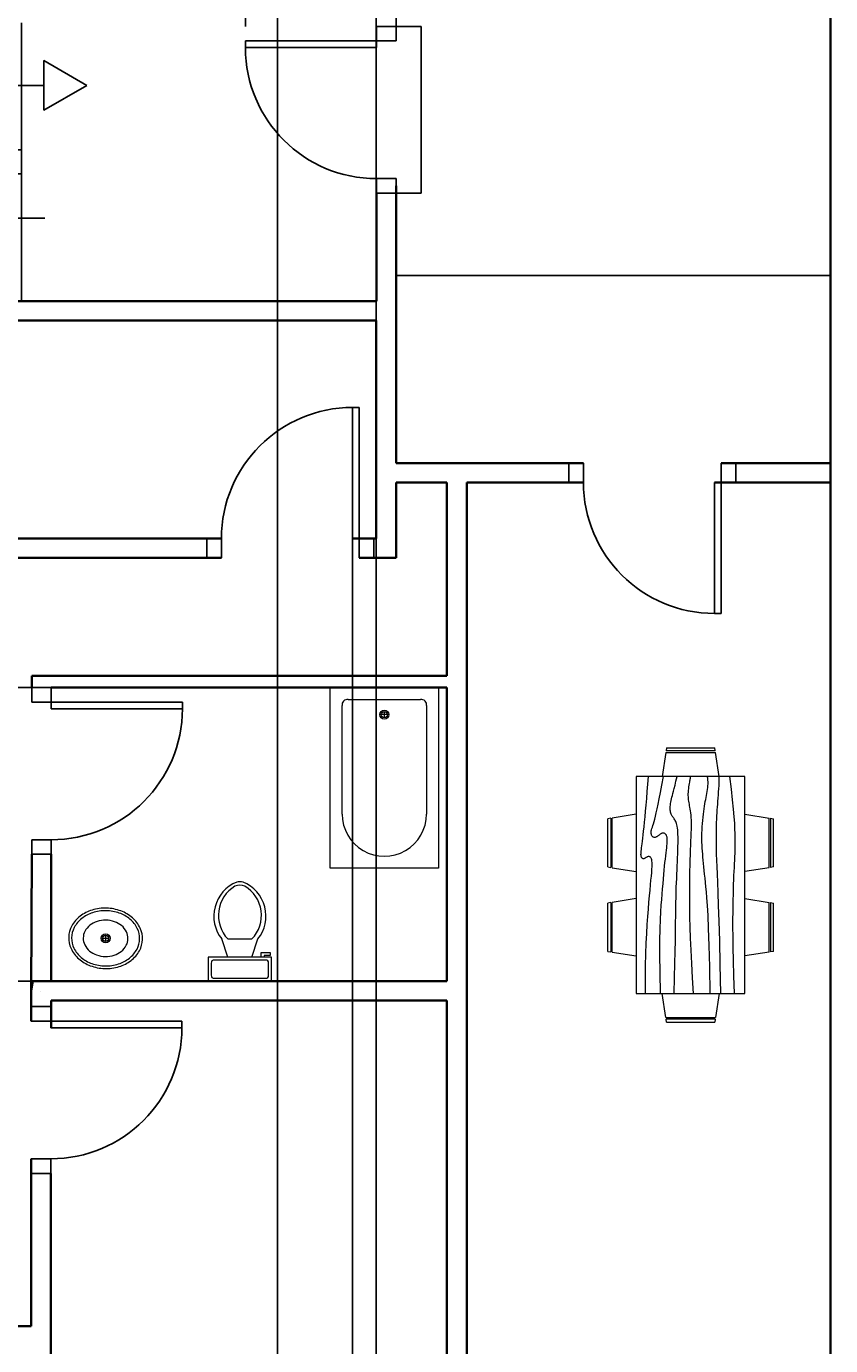
# Model space of a CAD drawing. Units: millimetres. Extents: x 31 to 27050, y -916 to 32407.
# Tile 3 of 7: x 6569 to 13341, y 5664 to 16782. Entities that reach past the tile are written whole.
import ezdxf

# ---------------------------------------------------------------- set-up
doc = ezdxf.new("R2010")
doc.units = ezdxf.units.MM
for name, color, linetype, lineweight in [('A-ANNO-DIMS', 2, 'Continuous', 18), ('A-DOOR', 3, 'Continuous', 25), ('A-FLOR-FIXT', 9, 'Continuous', 18), ('A-FLOR-STRS', 7, 'Continuous', 25), ('A-FURN', 8, 'Continuous', 13), ('A-WALL', 7, 'Continuous', 35)]:
    doc.layers.add(name, color=color, linetype=linetype, lineweight=lineweight)
doc.styles.get("Standard").update_dxf_attribs({"font": 'arial.ttf'})
doc.dimstyles.get("Standard").update_dxf_attribs({"dimtxt": 0.18, "dimasz": 0.18, "dimexe": 0.18, "dimexo": 0.0625, "dimgap": 0.09, "dimtad": 0, "dimtih": 1, "dimtoh": 1, "dimdec": 4, "dimzin": 0, "dimdsep": 46, "dimtxsty": 'Standard', "dimcen": 0.09, "dimadec": 0, "dimazin": 0, "dimtfac": 1, "dimtdec": 4, "dimtofl": 0, "dimtmove": 0, "dimatfit": 3, "dimfxl": 1, "dimtolj": 1, "dimtzin": 0, "dimarcsym": 0})

# ---------------------------------------------------------------- blocks, each defined once
blk = doc.blocks.new('Bath Tub - 26 x 60 in.')
for p, q in [((9, -17), (9, -19)), ((8, -18), (10, -18))]:
    blk.add_line(p, q)
blk.add_lwpolyline([(0, -36), (0, 0), (60, 0), (60, -36)], close=True)
for points in [[(6, -4), (42, -4)], [(4, -30), (4, -6)], [(42, -32), (6, -32)]]:
    blk.add_lwpolyline(points)
for radius in [1.5, 1]:
    blk.add_circle((9, -18), radius)
for centre, radius, start, end in [((5.75, -5.75), 1.767766999999999, 81.86989999999999, 188.1301), ((42, -18), 14, 270, 90), ((5.75, -30.25), 1.767766999999999, 171.8699, 278.1301)]:
    blk.add_arc(centre, radius, start, end)
blk = doc.blocks.new('Sink - Oval top')
for p, q in [((-1, 0), (1, 0)), ((0, 1), (0, -1))]:
    blk.add_line(p, q)
for points in [[(-12.23371880354079, 0.3941914712607968, 0.1176342565883263), (-11.46456229543957, -3.361933235489118, 0.104469279667093), (-8.878748691070427, -6.803541973650567, 0.0900157896014849), (-5.082757700676665, -9.072309807490512, 0.0819199491592185), (-0.3227280122732736, -10.01585280257211, 0.0819199491592091), (4.488169920880977, -9.380701564817912, 0.0900157896014801), (8.422342359155778, -7.36101289847943, 0.1044692796670922), (11.22435122606941, -4.093009071543406, 0.1176342565883338), (12.23371880354091, -0.3941914712607968, 0.1176342565883057), (11.46456229543992, 3.361933235488777, 0.1044692796670849), (8.878748691070427, 6.803541973650567, 0.0900157896014884), (5.082757700676324, 9.072309807490681, 0.0819199491592058), (0.3227280122732736, 10.01585280257211, 0.081919949159207), (-4.488169920880864, 9.380701564817969, 0.0900157896014802), (-8.422342359155778, 7.36101289847943, 0.1044692796670951), (-11.22435122606919, 4.093009071543633, 0.1176342565883402)], [(-11.28627986850119, 0.1590597164737346, 0.1186217001864142), (-10.51590095791209, -3.253161772358112, 0.1046781721811095), (-8.071803350560115, -6.358618019863342, 0.0895620664691738), (-4.537699193222351, -8.366971929609804, 0.0811846988912177), (-0.1289739026695997, -9.15150355811437, 0.0811846988912276), (4.300109150126218, -8.491524865184601, 0.0895620664691798), (7.889406708212618, -6.583562428127606, 0.1046781721811044), (10.42004782883111, -3.548216131892445, 0.1186217001864013), (11.28627986850119, -0.1590597164736209, 0.1186217001863945), (10.51590095791221, 3.253161772357998, 0.1046781721811069), (8.071803350560115, 6.358618019863342, 0.0895620664691756), (4.537699193222124, 8.366971929609917, 0.081184698891216), (0.1289739026695997, 9.151503558114428, 0.0811846988912142), (-4.300109150125877, 8.491524865184829, 0.0895620664691747), (-7.889406708212618, 6.583562428127606, 0.1046781721811045), (-10.42004782883111, 3.548216131892445, 0.1186217001863946)], [(-7.420452389032902, 0.0829876781601797, 0.1182825673856775), (-6.907065465214486, -2.1674649380775, 0.1046074595377274), (-5.294791470712084, -4.209988192029413, 0.0897179636260996), (-2.966599981142508, -5.528122152688069, 0.0814360825277113), (-0.0675135187855176, -6.036810076758797, 0.0814360825277218), (2.84222437824053, -5.593085960977873, 0.0897179636261315), (5.199312936802016, -4.327350491993342, 0.1046074595376878), (6.85686365682659, -2.321395784920355, 0.1182825673856714), (7.420452389033016, -0.0829876781601797, 0.1182825673856961), (6.907065465214486, 2.167464938077614, 0.1046074595377135), (5.294791470712084, 4.209988192029413, 0.0897179636261265), (2.966599981142621, 5.528122152687842, 0.0814360825277426), (0.0675135187855176, 6.036810076758797, 0.0814360825277225), (-2.842224378240644, 5.593085960977873, 0.0897179636261212), (-5.199312936802016, 4.327350491993342, 0.1046074595377049), (-6.856863656826476, 2.321395784920355, 0.1182825673856712)]]:
    blk.add_lwpolyline(points, format="xyb", close=True)
for radius in [1.5, 1]:
    blk.add_circle((0, 0), radius)
blk = doc.blocks.new('Toilet - top')
for p, q in [((9.5, -6), (9.5, -2)), ((-10, -8.5), (-8, -8.5)), ((-10, -9.5), (-10, -8.5)), ((-8, -8.5), (-8, -8)), ((-7, -8), (-7, -9.5)), ((-4, -8), (-6, -14)), ((4, -8), (6, -14)), ((-7, -9.5), (-10, -9.5)), ((4, -14), (-4, -14))]:
    blk.add_line(p, q)
blk.add_lwpolyline([(10.5, -8), (10.5, 0), (-10.5, 0), (-10.5, -8)], close=True)
for points in [[(-9.5, -2), (-9.5, -6)], [(8.5, -1), (-8.5, -1)], [(-8.5, -7), (8.5, -7)]]:
    blk.add_lwpolyline(points)
for centre, radius, start, end in [((-8.625, -1.875), 0.8838834999999999, 81.86989999999999, 188.1301), ((8.625, -1.875), 0.8838834999999999, 351.8699, 98.13009999999998), ((-8.625, -6.125), 0.8838834999999999, 171.869898, 278.1301), ((8.625, -6.125), 0.8838834999999999, 261.8699, 8.130099999999993), ((3.519562435188956, -21.58049502388982), 12.16902005083646, 141.4691096810948, 247.9714346835576), ((4.199957580658807, -21.81740929088453), 11.3291791325804, 136.3677254423718, 238.946823937405), ((-3.519499936778316, -21.58047137067522), 12.16903423757823, 292.0284332733152, 38.53070636800453), ((-4.199890672038477, -21.81738596564128), 11.32918622148567, 301.0530065773863, 43.63209216694732), ((2.09660981727e-05, -27.87646475467881), 4, 245.7318247449371, 294.2681740488959), ((2.09415214183e-05, -28.99996806116075), 4, 254.8605283244437, 285.1394707718433)]:
    blk.add_arc(centre, radius, start, end)
blk = doc.blocks.new('Dining Set - 36 x 72 in.')
for p, q in [((-22, 27.5), (-22.15620000000001, 26.50042)), ((-5.841600000000028, 26.5), (-22.15340000000003, 26.5)), ((-22, 27.5), (-6, 27.5)), ((-5.843700000000012, 26.49966), (-6, 27.5)), ((6, 27.5), (5.843799999999987, 26.50042)), ((22.15839999999997, 26.5), (5.846599999999966, 26.5)), ((6, 27.5), (22, 27.5)), ((22.15629999999999, 26.49966), (22, 27.5)), ((-22.23430000000002, 26.00059), (-23.48470000000003, 17.99762)), ((-22.23040000000003, 26), (-5.760800000000017, 26)), ((-4.515199999999992, 17.99762), (-5.765500000000031, 25.99926)), ((5.765699999999981, 26.00059), (4.515299999999967, 17.99762)), ((5.769599999999968, 26), (22.23919999999998, 26)), ((23.48480000000001, 17.99762), (22.23449999999997, 25.99926)), ((36, 18), (-36, 18)), ((-36, 18), (-36, -18)), ((36, -18), (36, 18)), ((-44.00060000000002, 8.234280000000002), (-35.99760000000003, 9.484740000000006)), ((44.00059999999996, 8.234280000000002), (35.99759999999998, 9.484740000000006)), ((-45.49999999999999, 8.000000000000004), (-44.50040000000001, 8.156170000000007)), ((-45.49999999999999, 8.000000000000004), (-45.49999999999999, -7.999999999999996)), ((-44.5, -8.15843), (-44.5, 8.153380000000002)), ((-44, 8.230410000000003), (-44, -8.239149999999999)), ((44, 8.230410000000003), (44, -8.239149999999999)), ((44.5, -8.15843), (44.5, 8.153380000000002)), ((45.49999999999999, 8.000000000000004), (44.50049999999999, 8.156170000000007)), ((45.49999999999999, 8.000000000000004), (45.49999999999999, -7.999999999999996)), ((-44.49970000000002, -8.156309999999994), (-45.49999999999999, -7.999999999999996)), ((-35.99760000000003, -9.484759999999998), (-43.9993, -8.234499999999993)), ((35.99759999999998, -9.484759999999998), (43.9993, -8.234499999999993)), ((44.49969999999995, -8.156309999999994), (45.49999999999999, -7.999999999999996)), ((-36, -18), (36, -18)), ((-22.23430000000002, -26.0006), (-23.48470000000003, -17.99762)), ((-4.515199999999992, -17.99762), (-5.765500000000031, -25.99928)), ((5.765699999999981, -26.0006), (4.515299999999967, -17.99762)), ((23.48480000000001, -17.99762), (22.23449999999997, -25.99928)), ((-22.23040000000003, -26), (-5.760800000000017, -26)), ((5.769599999999968, -26), (22.23919999999998, -26)), ((-22, -27.5), (-22.15620000000001, -26.50044)), ((-5.841600000000028, -26.5), (-22.15340000000003, -26.5)), ((-22, -27.5), (-6, -27.5)), ((-5.843700000000012, -26.49967), (-6, -27.5)), ((6, -27.5), (5.843799999999987, -26.50044)), ((22.15839999999997, -26.5), (5.846599999999966, -26.5)), ((6, -27.5), (22, -27.5)), ((22.15629999999999, -26.49967), (22, -27.5))]:
    blk.add_line(p, q)
for points in [[(-36, 15), (-31.17720000000003, 14.97754), (-26.80790000000002, 14.91406), (-22.85380000000003, 14.81543), (-19.27600000000001, 14.6875), (-16.03620000000001, 14.53613), (-13.09570000000002, 14.36718), (-10.41590000000002, 14.18652), (-7.958300000000008, 14), (-5.690400000000011, 13.81315), (-3.603499999999996, 13.63021), (-1.695400000000006, 13.45508), (0.0364999999999896, 13.29166), (1.594499999999982, 13.14388), (2.981099999999969, 13.01562), (4.198800000000005, 12.9108), (5.25, 12.83333), (6.139299999999991, 12.78613), (6.880200000000002, 12.76823), (7.488299999999981, 12.77767), (7.979199999999991, 12.8125), (8.368499999999983, 12.87077), (8.671899999999994, 12.95052), (8.904899999999998, 13.0498), (9.083300000000008, 13.16666), (9.220499999999959, 13.29899000000001), (9.32159999999999, 13.44401), (9.389499999999998, 13.59879), (9.427099999999996, 13.76041), (9.437299999999993, 13.92594), (9.423200000000008, 14.09245), (9.387499999999989, 14.257), (9.333300000000008, 14.41666), (9.263800000000003, 14.56917), (9.183600000000013, 14.71484), (9.097499999999968, 14.85465), (9.010400000000004, 14.98958), (8.92719999999997, 15.12060000000001), (8.852899999999975, 15.2487), (8.79219999999998, 15.37483), (8.75, 15.5), (8.730500000000006, 15.62467), (8.734399999999994, 15.74739), (8.761699999999962, 15.86621), (8.8125, 15.97916), (8.886699999999962, 16.08431), (8.984399999999994, 16.17968), (9.105500000000006, 16.26334), (9.25, 16.33333), (9.418900000000008, 16.38802), (9.617199999999968, 16.42708), (9.850599999999986, 16.45052), (10.125, 16.45833), (10.44630000000001, 16.45052), (10.82029999999997, 16.42708), (11.25290000000001, 16.38802), (11.75, 16.33333), (12.3184, 16.26318), (12.96940000000001, 16.17838), (13.7151, 16.07991), (14.5677, 15.96875), (15.53949999999997, 15.84586), (16.64259999999996, 15.71224), (17.88929999999999, 15.56884), (19.29169999999999, 15.41666), (20.85899999999998, 15.25667), (22.58789999999999, 15.08984), (24.47210000000001, 14.91715), (26.5052, 14.73958), (28.68090000000001, 14.5581), (30.99289999999996, 14.3737), (33.43469999999996, 14.18733), (36, 14)], [(-36, 10), (-28.97660000000002, 10.14274000000001), (-23.17250000000001, 10.20442), (-18.42410000000001, 10.19775), (-14.5677, 10.13541), (-11.43990000000002, 10.03011), (-8.87700000000001, 9.894530000000007), (-6.715399999999988, 9.741370000000005), (-4.791699999999991, 9.58333), (-2.96980000000002, 9.43082), (-1.224600000000009, 9.285150000000005), (0.4414999999999623, 9.14534), (2.02600000000001, 9.010410000000004), (3.526599999999973, 8.879390000000004), (4.940799999999967, 8.751300000000004), (6.265999999999962, 8.625160000000005), (7.5, 8.500000000000004), (8.641099999999994, 8.375490000000003), (9.691399999999987, 8.253900000000005), (10.65379999999999, 8.13818), (11.53120000000001, 8.031250000000004), (12.32669999999996, 7.936030000000005), (13.043, 7.85547), (13.68309999999997, 7.792480000000001), (14.25, 7.750000000000003), (14.74709999999999, 7.730300000000003), (15.17969999999997, 7.733070000000001), (15.55369999999999, 7.757320000000003), (15.875, 7.80208), (16.14940000000001, 7.866370000000006), (16.38279999999997, 7.94922), (16.58109999999999, 8.04964), (16.75, 8.166660000000004), (16.89439999999996, 8.29915), (17.01429999999999, 8.445310000000003), (17.1089, 8.603190000000001), (17.17709999999999, 8.77083), (17.21799999999996, 8.946290000000001), (17.2305, 9.127600000000005), (17.21369999999996, 9.312820000000006), (17.16669999999999, 9.500000000000004), (17.08949999999999, 9.687500000000004), (16.98699999999996, 9.875000000000004), (16.86489999999998, 10.0625), (16.72919999999999, 10.25), (16.5856, 10.4375), (16.44009999999997, 10.625), (16.29849999999999, 10.8125), (16.16669999999999, 11), (16.05000000000001, 11.18733), (15.95179999999999, 11.3737), (15.8752, 11.5581), (15.8229, 11.73958), (15.798, 11.91715), (15.80340000000001, 12.08984), (15.84199999999998, 12.25667), (15.91669999999999, 12.41666), (16.02949999999998, 12.56836), (16.17840000000001, 12.70833), (16.3605, 12.83268), (16.5729, 12.9375), (16.8127, 13.01888000000001), (17.07679999999999, 13.07291), (17.36250000000001, 13.0957), (17.66669999999999, 13.08333), (17.98939999999999, 13.03312), (18.34179999999998, 12.94726), (18.7382, 12.82918), (19.1927, 12.68229), (19.71949999999998, 12.51001), (20.33269999999999, 12.31575), (21.04649999999998, 12.10294), (21.875, 11.875), (22.83569999999997, 11.63354), (23.95900000000001, 11.37304), (25.27859999999999, 11.08618), (26.82819999999998, 10.76562), (28.64139999999998, 10.40405), (30.75200000000001, 9.994140000000005), (33.1936, 9.528560000000002), (36, 9.000000000000004)], [(-36, 5.500000000000003), (-30.71570000000003, 5.334800000000004), (-26.06900000000002, 5.20963), (-21.99459999999999, 5.11767), (-18.42709999999999, 5.05208), (-15.30090000000001, 5.006020000000003), (-12.55080000000004, 4.972650000000005), (-10.1112, 4.945150000000001), (-7.916699999999991, 4.916660000000003), (-5.908999999999991, 4.881670000000003), (-4.058600000000012, 4.839840000000005), (-2.342899999999985, 4.792150000000003), (-0.7395999999999959, 4.73958), (0.7738999999999692, 4.683100000000006), (2.21999999999997, 4.623700000000003), (3.621299999999962, 4.562330000000006), (5, 4.500000000000003), (6.37299999999999, 4.437820000000005), (7.734399999999993, 4.377600000000004), (9.072299999999984, 4.321290000000001), (10.375, 4.27083), (11.63089999999999, 4.228190000000001), (12.8281, 4.195310000000002), (13.95509999999996, 4.17415), (15, 4.166660000000003), (15.95400000000001, 4.174480000000006), (16.81899999999996, 4.197910000000003), (17.6001, 4.236980000000006), (18.30209999999999, 4.291660000000003), (18.92989999999997, 4.361980000000006), (19.48829999999998, 4.447910000000003), (19.98230000000001, 4.549480000000006), (20.41669999999999, 4.666660000000003), (20.79689999999999, 4.798990000000006), (21.1302, 4.944010000000002), (21.42449999999997, 5.098790000000004), (21.6875, 5.260410000000003), (21.92709999999999, 5.42594), (22.15109999999999, 5.592450000000003), (22.36719999999997, 5.757000000000001), (22.58339999999998, 5.916660000000003), (22.80649999999997, 6.068680000000004), (23.04039999999998, 6.210930000000001), (23.28789999999998, 6.341470000000004), (23.5521, 6.45833), (23.83580000000001, 6.559570000000004), (24.142, 6.643230000000006), (24.4735, 6.707350000000001), (24.83339999999998, 6.750000000000003), (25.2235, 6.76969), (25.642, 6.766920000000002), (26.08580000000001, 6.74267), (26.5521, 6.697910000000003), (27.03789999999998, 6.633620000000004), (27.54039999999998, 6.550780000000006), (28.05649999999997, 6.450360000000006), (28.58339999999998, 6.33333), (29.12419999999997, 6.19987), (29.70709999999997, 6.046870000000001), (30.36609999999996, 5.870440000000005), (31.1354, 5.666660000000003), (32.04929999999996, 5.431640000000005), (33.142, 5.161460000000001), (34.44749999999999, 4.852210000000003), (36, 4.500000000000003)], [(-36, -0.9999999999999964), (-30.79150000000004, -0.6590999999999987), (-26.01949999999999, -0.3821599999999954), (-21.65190000000001, -0.1628399999999992), (-17.65629999999999, 0.0052100000000017), (-14.00049999999999, 0.1283300000000018), (-10.65230000000002, 0.2128900000000051), (-7.579600000000027, 0.2652200000000029), (-4.75, 0.2916600000000038), (-2.134000000000014, 0.2979300000000045), (0.2878000000000043, 0.287110000000002), (2.5317, 0.2616300000000002), (4.614599999999995, 0.2239600000000017), (6.552899999999965, 0.1765100000000039), (8.363299999999981, 0.1217400000000062), (10.06229999999999, 0.0620900000000013), (11.66669999999999, 3.6e-15), (13.18989999999996, -0.0620099999999972), (14.63409999999999, -0.1210999999999949), (15.9982, -0.174319999999998), (17.28129999999999, -0.2187499999999964), (18.48230000000001, -0.2514699999999941), (19.6003, -0.2695299999999996), (20.6343, -0.2700199999999988), (21.58339999999999, -0.2499999999999964), (22.44810000000001, -0.2076799999999999), (23.23570000000001, -0.1458399999999962), (23.95490000000001, -0.0683599999999949), (24.6146, 0.0208300000000001), (25.2235, 0.1178400000000046), (25.79039999999998, 0.2187500000000035), (26.32409999999999, 0.3196600000000025), (26.83339999999998, 0.4166600000000038), (27.32650000000001, 0.5061800000000041), (27.80989999999997, 0.5859300000000012), (28.2894, 0.6539700000000046), (28.77089999999999, 0.7083300000000002), (29.26009999999997, 0.7470700000000045), (29.76299999999998, 0.7682300000000062), (30.28550000000001, 0.7698500000000017), (30.83339999999998, 0.7500000000000036), (31.40879999999999, 0.707840000000001), (31.99939999999998, 0.6471300000000006), (32.589, 0.5727500000000028), (33.16149999999999, 0.4895800000000002), (33.70079999999996, 0.402500000000007), (34.19079999999997, 0.3164000000000051), (34.61529999999999, 0.2361600000000017), (34.95839999999998, 0.1666600000000038), (35.20990000000001, 0.1116500000000009), (35.38479999999998, 0.0703100000000028), (35.50399999999996, 0.0406900000000015), (35.58859999999999, 0.0208300000000001), (35.65940000000001, 0.0087900000000012), (35.73769999999996, 0.0026000000000046), (35.8442, 0.0003200000000056), (36, 3.6e-15)], [(-36, -6.499999999999996), (-27.18430000000001, -6.312669999999993), (-20.084, -6.126299999999996), (-14.46899999999999, -5.941899999999993), (-10.10939999999999, -5.760419999999999), (-6.77520000000004, -5.582849999999996), (-4.236300000000028, -5.410159999999994), (-2.262900000000001, -5.243329999999996), (-0.625, -5.083339999999996), (0.8707999999999742, -4.930989999999997), (2.271500000000003, -4.786459999999994), (3.587199999999995, -4.649739999999997), (4.828100000000006, -4.520839999999996), (6.004599999999982, -4.399739999999997), (7.127000000000009, -4.286459999999994), (8.205299999999966, -4.180989999999997), (9.25, -4.083339999999996), (10.27049999999997, -3.993819999999995), (11.27339999999998, -3.914069999999998), (12.2647, -3.846029999999995), (13.25, -3.791669999999999), (14.23539999999997, -3.752929999999995), (15.22659999999996, -3.731769999999993), (16.22949999999997, -3.730149999999998), (17.25, -3.749999999999996), (18.2912, -3.792479999999994), (19.3451, -3.855469999999993), (20.40089999999998, -3.936039999999994), (21.4479, -4.031249999999996), (22.47539999999998, -4.138189999999998), (23.47269999999998, -4.253909999999994), (24.4289, -4.375489999999995), (25.33339999999999, -4.499999999999996), (26.17849999999999, -4.624919999999999), (26.96940000000001, -4.749349999999996), (27.71449999999999, -4.872809999999997), (28.4219, -4.994789999999998), (29.09999999999996, -5.114829999999994), (29.75720000000001, -5.232419999999994), (30.40159999999997, -5.347089999999997), (31.04169999999999, -5.458339999999996), (31.68369999999999, -5.564369999999993), (32.32619999999997, -5.658209999999993), (32.9658, -5.731529999999995), (33.59899999999999, -5.776039999999998), (34.22239999999999, -5.783449999999998), (34.83269999999999, -5.745449999999994), (35.4264, -5.653729999999999), (36, -5.499999999999996)], [(-36, -9.999999999999996), (-26.40219999999999, -9.812989999999996), (-18.46750000000003, -9.628909999999994), (-11.9839, -9.450689999999998), (-6.739599999999995, -9.281249999999996), (-2.522600000000011, -9.123539999999995), (0.8788999999999872, -8.980469999999993), (3.676899999999989, -8.854979999999994), (6.083300000000008, -8.749999999999996), (8.276700000000005, -8.667649999999998), (10.30209999999999, -8.606769999999994), (12.1712, -8.565429999999996), (13.89580000000001, -8.54167), (15.48759999999998, -8.533529999999995), (16.95830000000001, -8.539069999999999), (18.31970000000001, -8.556319999999994), (19.58339999999998, -8.583339999999996), (20.76159999999999, -8.618409999999994), (21.86849999999998, -8.660809999999994), (22.91879999999998, -8.710039999999996), (23.9271, -8.765629999999998), (24.90809999999999, -8.827069999999996), (25.87629999999996, -8.89388), (26.84649999999999, -8.96558), (27.83339999999999, -9.04167), (28.84739999999999, -9.121179999999997), (29.88279999999998, -9.201169999999994), (30.93000000000001, -9.278239999999993), (31.97919999999999, -9.348959999999995), (33.02049999999997, -9.409909999999998), (34.04429999999996, -9.45768), (35.04069999999996, -9.488849999999996), (36, -9.499999999999996)], [(-36, -14.5), (-30.0881, -14.33512999999999), (-25.03320000000002, -14.21224), (-20.7312, -14.12646999999999), (-17.0781, -14.07292), (-13.97000000000003, -14.04670999999999), (-11.30270000000001, -14.04296999999999), (-8.972399999999993, -14.05680999999999), (-6.875, -14.08333999999999), (-4.922400000000038, -14.11832999999999), (-3.09050000000002, -14.16015999999999), (-1.370900000000006, -14.20784999999999), (0.2447999999999979, -14.26042), (1.764700000000004, -14.31689999999999), (3.197299999999984, -14.37629999999999), (4.550700000000006, -14.43766999999999), (5.833300000000008, -14.5), (7.055399999999963, -14.5621), (8.235000000000014, -14.62174999999999), (9.392200000000003, -14.67652), (10.54689999999999, -14.72395999999999), (11.7192, -14.76164), (12.92899999999997, -14.78711), (14.19649999999996, -14.79794), (15.54169999999999, -14.79167), (16.99329999999998, -14.76423999999999), (18.61519999999996, -14.70508), (20.48039999999998, -14.60197), (22.66149999999999, -14.44270999999999), (25.2312, -14.21509), (28.26240000000002, -13.90689999999999), (31.8277, -13.50594), (36, -13)]]:
    blk.add_lwpolyline(points)
blk = doc.blocks.new('DOOR-SINGLE-1104')
for p, q in [((56.41678681898429, 1104.337341461596), (-7.18501e-11, 1104.337341461596)), ((-7.18501e-11, 1104.337341461596), (-7.18501e-11, 3.638e-12)), ((56.41678681898429, 7.276e-12), (56.41678681898429, 1104.337341461596)), ((-1226.913698425656, -163.8831223050438), (-1226.913698425656, 3.638e-12)), ((-1104.337341461589, 3.638e-12), (-1226.913698425656, 7.276e-12)), ((-1104.337341461589, 3.638e-12), (-1104.337341461589, -163.8831223050438)), ((-7.18501e-11, 3.638e-12), (56.41678681898429, 7.276e-12)), ((56.41678681898429, -163.8831223050438), (56.41678681898429, 3.638e-12)), ((56.41678681898429, 3.638e-12), (178.9931437830519, 3.638e-12)), ((178.9931437830519, 3.638e-12), (178.9931437830519, -163.8831223050438)), ((-1104.337341461589, -163.8831223050438), (-1226.913698425656, -163.8831223050438)), ((178.9931437830519, -163.8831223050438), (56.41678681898429, -163.8831223050438))]:
    blk.add_line(p, q)
blk.add_arc((0, 3.638e-12), 1104.337341461589, 90, 180)
blk = doc.blocks.new('STAIR-RETURN-2400')
for p, q in [((9.095e-13, 2345.636859649549), (9.095e-13, -1.819e-12)), ((200.0000000000009, 2345.636859649549), (200.0000000000009, -1.819e-12)), ((400.0000000000008, 2345.636859649549), (400.0000000000008, -1.819e-12)), ((600.0000000000008, 2345.636859649549), (600.0000000000008, -1.819e-12)), ((800.0000000000008, 2345.636859649552), (800.0000000000008, 1.819e-12)), ((1000.000000000001, 2345.636859649556), (1000.000000000001, 5.457e-12)), ((1200.000000000001, 2345.636859649556), (1200.000000000001, 5.457e-12)), ((1400.000000000001, 2345.636859649556), (1400.000000000001, 5.457e-12)), ((1600.000000000001, 2345.636859649559), (1600.000000000001, 9.0949e-12)), ((1800.000000000001, 2345.636859649559), (1800.000000000001, 9.0949e-12)), ((2000.000000000001, 2345.636859649559), (2000.000000000001, 9.0949e-12)), ((2200.000000000001, 2345.636859649563), (2200.000000000001, 1.27329e-11)), ((2400.000000000001, 2345.636859649563), (2400.000000000001, 1.27329e-11)), ((-415.9249645337103, 697.4958917418807), (-415.9249645337103, 1817.654410237617)), ((-415.9249645337103, 1817.654410237617), (2588.331988211024, 1817.654410237617)), ((9.095e-13, 1172.818429824772), (9.095e-13, 1272.818429824772)), ((9.095e-13, 1272.818429824772), (2400.000000000001, 1272.818429824774)), ((2400.000000000001, 1272.818429824774), (2400.000000000001, 1072.818429824774)), ((2400.000000000001, 1072.818429824774), (9.095e-13, 1072.818429824774)), ((2597.09055342863, 697.4958917418807), (-415.9249645337103, 697.4958917418807))]:
    blk.add_line(p, q)
blk.add_lwpolyline([(2948.607295106225, 1817.654410237617), (2588.331988211024, 2025.65945565594), (2588.331988211024, 1609.649364819299)], close=True)
blk = doc.blocks.new('*D16')
at = {"layer": 'A-ANNO-DIMS', "color": 0, "lineweight": -2, "transparency": 16777216}
for p, q in [((9681.744557342236, 16781.90361905769), (9892.748083673547, 16781.90361905769)), ((9892.568083673546, 16781.72361905769), (9892.568083673546, 16079.13332892196)), ((9892.568083673546, 15376.17677684898), (9892.568083673546, 16078.76706698471)), ((9681.744557342237, 15375.99677684898), (9892.748083673547, 15375.99677684898))]:
    blk.add_line(p, q, dxfattribs=at)
at = {"layer": 'A-ANNO-DIMS', "color": 0, "transparency": 16777216}
for points in [[(9892.538083673546, 16781.72361905769), (9892.598083673547, 16781.72361905769), (9892.568083673546, 16781.90361905769)], [(9892.538083673546, 15376.17677684898), (9892.598083673547, 15376.17677684898), (9892.568083673546, 15375.99677684898)]]:
    blk.add_solid(points, dxfattribs=at)
at = {"layer": 'Defpoints', "color": 0, "transparency": 16777216}
for p in [(9681.682057342236, 16781.90361905769), (9892.568083673546, 16781.90361905769), (9681.682057342237, 15375.99677684898)]:
    blk.add_point(p, dxfattribs=at)
at = {"layer": 'A-ANNO-DIMS', "color": 0, "transparency": 16777216, "insert": (9892.568083673552, 16078.95019795333), "char_height": 0.18, "attachment_point": 5}
blk.add_mtext('\\A1;DOOR 1406 TYP.', dxfattribs=at)
blk = doc.blocks.new('*D17')
at = {"layer": 'A-ANNO-DIMS', "color": 0, "lineweight": -2, "transparency": 16777216}
for p, q in [((8413.461593575592, 16781.96611905768), (8413.461593575592, 16992.96964538898)), ((8413.641593575592, 16992.78964538898), (9046.912357518939, 16992.78964538899)), ((9681.502057342232, 16992.78964538899), (9048.231293398885, 16992.78964538899)), ((9681.682057342232, 16781.96611905768), (9681.682057342232, 16992.96964538899))]:
    blk.add_line(p, q, dxfattribs=at)
at = {"layer": 'A-ANNO-DIMS', "color": 0, "transparency": 16777216}
for points in [[(8413.641593575592, 16992.81964538898), (8413.641593575592, 16992.75964538898), (8413.461593575592, 16992.78964538898)], [(9681.502057342232, 16992.81964538899), (9681.502057342232, 16992.75964538899), (9681.682057342232, 16992.78964538899)]]:
    blk.add_solid(points, dxfattribs=at)
at = {"layer": 'Defpoints', "color": 0, "transparency": 16777216}
for p in [(8413.461593575592, 16992.78964538898), (8413.461593575592, 16781.90361905768), (9681.682057342232, 16781.90361905768)]:
    blk.add_point(p, dxfattribs=at)
at = {"layer": 'A-ANNO-DIMS', "color": 0, "transparency": 16777216, "insert": (9047.571825458914, 16992.78964538899), "char_height": 0.18, "attachment_point": 5}
blk.add_mtext('\\A1;1268 TYP.', dxfattribs=at)
blk = doc.blocks.new('*D64')
at = {"layer": 'A-ANNO-DIMS', "color": 0, "lineweight": -2, "transparency": 16777216}
for p, q in [((6778.040612000004, 11210.336516), (5198.923112000002, 11210.336516)), ((5199.103112000003, 11210.156516), (5199.103112000003, 9972.897271637792)), ((5199.103112000003, 8735.274221000001), (5199.103112000003, 9972.533465362214)), ((6778.040612000004, 8735.094221000001), (5198.923112000003, 8735.094221000001))]:
    blk.add_line(p, q, dxfattribs=at)
at = {"layer": 'A-ANNO-DIMS', "color": 0, "transparency": 16777216}
for points in [[(5199.073112000003, 11210.156516), (5199.133112000002, 11210.156516), (5199.103112000003, 11210.336516)], [(5199.073112000004, 8735.274221000001), (5199.133112000003, 8735.274221000001), (5199.103112000003, 8735.094221000001)]]:
    blk.add_solid(points, dxfattribs=at)
at = {"layer": 'Defpoints', "color": 0, "transparency": 16777216}
for p in [(5199.103112000003, 11210.336516), (6778.103112000003, 11210.336516), (6778.103112000003, 8735.094221000001)]:
    blk.add_point(p, dxfattribs=at)
at = {"layer": 'A-ANNO-DIMS', "color": 0, "transparency": 16777216, "insert": (5199.103112000005, 9972.7153685), "char_height": 0.18, "attachment_point": 5}
blk.add_mtext('\\A1;2475', dxfattribs=at)
blk = doc.blocks.new('*D68')
at = {"layer": 'A-ANNO-DIMS', "color": 0, "lineweight": -2, "transparency": 16777216}
for p, q in [((9681.682057000002, 13102.073129), (9681.682057000002, 14681.190629)), ((9681.862057, 14681.010629), (11510.77480004775, 14681.010629)), ((13340.405333, 14681.010629), (11511.49258995225, 14681.010629)), ((13340.585333, 13102.073129), (13340.585333, 14681.190629))]:
    blk.add_line(p, q, dxfattribs=at)
at = {"layer": 'A-ANNO-DIMS', "color": 0, "transparency": 16777216}
for points in [[(9681.862057, 14681.040629), (9681.862057, 14680.980629), (9681.682057000002, 14681.010629)], [(13340.405333, 14681.040629), (13340.405333, 14680.980629), (13340.585333, 14681.010629)]]:
    blk.add_solid(points, dxfattribs=at)
at = {"layer": 'Defpoints', "color": 0, "transparency": 16777216}
for p in [(13340.585333, 14681.010629), (9681.682057000002, 13102.010629), (13340.585333, 13102.010629)]:
    blk.add_point(p, dxfattribs=at)
at = {"layer": 'A-ANNO-DIMS', "color": 0, "transparency": 16777216, "insert": (11511.133695, 14681.010629), "char_height": 0.18, "attachment_point": 5}
blk.add_mtext('\\A1;3659', dxfattribs=at)
blk = doc.blocks.new('*D74')
at = {"layer": 'A-ANNO-DIMS', "color": 0, "lineweight": -2, "transparency": 16777216}
for p, q in [((8684.522829, 19025.373224), (8684.522828999998, -915.5318640000004)), ((9513.331407, 19025.373224), (9513.331407, -915.5318640000004)), ((8684.702829, -915.3518639999999), (9098.533107085947, -915.3518639999999)), ((9513.151406999998, -915.3518639999999), (9099.321128914047, -915.3518639999999))]:
    blk.add_line(p, q, dxfattribs=at)
at = {"layer": 'A-ANNO-DIMS', "color": 0, "transparency": 16777216}
for points in [[(8684.702829, -915.321864), (8684.702829, -915.381864), (8684.522828999998, -915.3518639999999)], [(9513.151406999998, -915.321864), (9513.151406999998, -915.381864), (9513.331407, -915.3518639999999)]]:
    blk.add_solid(points, dxfattribs=at)
at = {"layer": 'Defpoints', "color": 0, "transparency": 16777216}
for p in [(8684.522829, 19025.435724), (9513.331407, 19025.435724), (8684.522828999998, -915.3518639999999)]:
    blk.add_point(p, dxfattribs=at)
at = {"layer": 'A-ANNO-DIMS', "color": 0, "transparency": 16777216, "insert": (9098.927117999998, -915.3518639999999), "char_height": 0.18, "attachment_point": 5}
blk.add_mtext('\\A1;828.8', dxfattribs=at)
blk = doc.blocks.new('*D75')
at = {"layer": 'A-ANNO-DIMS', "color": 0, "lineweight": -2, "transparency": 16777216}
for p, q in [((9315.42813, 12465.681171), (9315.42813, -915.5318640000004)), ((9513.331407, 12465.681171), (9513.331407, -915.5318640000004)), ((9315.60813, -915.3518639999999), (9413.994352401773, -915.3518639999999)), ((9513.151407, -915.3518639999999), (9414.765184598225, -915.3518639999999))]:
    blk.add_line(p, q, dxfattribs=at)
at = {"layer": 'A-ANNO-DIMS', "color": 0, "transparency": 16777216}
for points in [[(9315.60813, -915.321864), (9315.60813, -915.381864), (9315.42813, -915.3518639999999)], [(9513.151407, -915.321864), (9513.151407, -915.381864), (9513.331407, -915.3518639999999)]]:
    blk.add_solid(points, dxfattribs=at)
at = {"layer": 'Defpoints', "color": 0, "transparency": 16777216}
for p in [(9315.42813, 12465.743671), (9513.331407, 12465.743671), (9513.331407, -915.3518639999999)]:
    blk.add_point(p, dxfattribs=at)
at = {"layer": 'A-ANNO-DIMS', "color": 0, "transparency": 16777216, "insert": (9414.379768499999, -915.3518639999999), "char_height": 0.18, "attachment_point": 5}
blk.add_mtext('\\A1;197.9', dxfattribs=at)

msp = doc.modelspace()

# ---------------------------------------------------------------- linework, layer by layer
at = {"layer": 'A-DOOR'}
for p, q in [((6778.103112139866, 11210.33651640691), (6614.219989834819, 11210.33651640691)), ((6773.905119419517, 8521.175884980112), (6610.021997114469, 8521.175884980112))]:
    msp.add_line(p, q, dxfattribs=at)
at = {"layer": 'A-WALL'}
for p, q in [((13340.58533261045, 13102.01062910059), (13340.58533261045, 17938.12750679554)), ((9517.798935037174, 15375.99677684899), (9517.798935037174, 14467.4249367068)), ((9681.682057342221, 14467.4249367068), (9681.682057342221, 15437.28495533102)), ((2757.34083568836, 14467.4249367068), (9517.798935037174, 14467.4249367068)), ((9681.682057342221, 14384.27405581066), (9681.682057342221, 14467.4249367068)), ((9681.682057342221, 14384.27405581066), (9681.682057342221, 13102.01062910059)), ((2925.691486399059, 14303.54181440175), (9513.331406631527, 14303.54181440175)), ((9513.331406631527, 14303.54181440175), (9513.331406631527, 12465.74367114626)), ((11259.57994150526, 13102.01062910059), (9681.682057342221, 13102.01062910059)), ((13340.58533261045, 13102.01062910059), (12420.33406978584, 13102.01062910059)), ((13340.58533261045, 12938.12750679554), (13340.58533261045, 13102.01062910059)), ((9681.682057342221, 12938.12750679554), (9681.682057342221, 12382.59279025013)), ((10110.02199711447, 12938.12750679554), (9681.682057342221, 12938.12750679554)), ((10110.02199711447, 12938.12750679554), (10110.02199711446, 11309.00881926711)), ((10278.37264782516, 12938.12750679554), (10278.37264782516, 827.5312586717337)), ((11259.57994150526, 12938.12750679554), (10278.37264782516, 12938.12750679554)), ((13340.58533261045, 12938.12750679554), (12363.91728296678, 12938.12750679554)), ((13340.58533261045, 827.5312586717337), (13340.58533261045, 12938.12750679554)), ((8211.090788713413, 12465.74367114626), (2925.691486399059, 12465.74367114627)), ((9513.331406631527, 12465.74367114626), (9315.428130174929, 12465.74367114626)), ((9681.682057342221, 12301.86054884122), (9681.682057342221, 12382.59279025013)), ((8211.090788713413, 12301.86054884122), (5781.707676021313, 12301.86054884121)), ((9593.894742127508, 12301.86054884122), (9371.844916993983, 12301.86054884122)), ((9593.894742127508, 12301.86054884122), (9681.682057342221, 12301.86054884122)), ((6614.219989834819, 11210.33651640691), (6614.219989834819, 11309.00881926711)), ((6614.219989834819, 11309.00881926711), (10110.02199711447, 11309.00881926711)), ((6778.103112139866, 11210.33651640691), (10110.02199711447, 11210.33651640691)), ((10110.02199711447, 11210.33651640691), (10110.02199711447, 8735.094220936826)), ((6614.219989834822, 9804.429674198203), (6610.021997114469, 8651.943340040685)), ((6778.103112139874, 9804.429674198203), (6778.103112139874, 8735.094220936826)), ((6610.021997114469, 8651.943340040685), (6610.021997114469, 8735.094220936828)), ((6610.021997114469, 8735.094220936828), (6690.58533261045, 8735.094220936826)), ((6610.021997114469, 8651.943340040685), (6622.148902538111, 8735.094220936828)), ((6690.58533261045, 8735.094220936826), (10110.02199711447, 8735.094220936826)), ((6610.021997114469, 8398.599528016042), (6610.021997114469, 8651.943340040685)), ((6690.58533261045, 8651.943340040685), (6690.58533261045, 8651.943340040685)), ((6778.372647825162, 8571.211098631777), (10110.02199711446, 8571.211098631771)), ((6778.372647825162, 8342.182741196984), (6778.372647825162, 8571.211098631777)), ((10110.02199711447, 8571.211098631777), (10110.02199711447, 827.5312586717337)), ((6610.021997114469, 5827.531258671733), (6610.021997114471, 7237.845399735471)), ((6773.905119419524, 7115.269042771405), (6778.372647825162, 827.5312586717337)), ((6302.191350742941, 5827.531258671733), (6610.021997114469, 5827.531258671733))]:
    msp.add_line(p, q, dxfattribs=at)

# ---------------------------------------------------------------- block references
at = {"layer": 'A-DOOR', "rotation": 90.00000000000006}
msp.add_blockref('DOOR-SINGLE-1104', (9517.798935037188, 16602.91047527463), dxfattribs=at)
at = {"layer": 'A-DOOR'}
msp.add_blockref('DOOR-SINGLE-1104', (9315.428130175002, 12465.74367114624), dxfattribs=at)
at = {"layer": 'A-DOOR', "extrusion": (0, 0, -1), "zscale": -1}
for p, rotation in [((-12363.91728296685, 12938.12750679555), 180), ((-6778.103112139851, 11031.34337262386), 90.00000000000028), ((-6773.905119419501, 8342.182741197055), 89.99999999999996)]:
    msp.add_blockref('DOOR-SINGLE-1104', p, dxfattribs=dict(at, rotation=rotation))
at = {"layer": 'A-FLOR-FIXT', "xscale": 25.4, "yscale": 25.4, "zscale": 25.4}
for name, p, rotation in [('Bath Tub - 26 x 60 in.', (10040.2342069835, 11210.33651640691), 270), ('Toilet - top', (8366.84177489248, 8735.094220936826), 180)]:
    msp.add_blockref(name, p, dxfattribs=dict(at, rotation=rotation))
msp.add_blockref('Sink - Oval top', (7236.106883122694, 9096.171958548497), dxfattribs=at)
at = {"layer": 'A-FLOR-STRS'}
msp.add_blockref('STAIR-RETURN-2400', (4128.594056532892, 14467.4249367068), dxfattribs=at)
at = {"layer": 'A-FURN', "xscale": 25.4, "yscale": 25.4, "zscale": 25.4, "rotation": 90}
msp.add_blockref('Dining Set - 36 x 72 in.', (12162.05807908132, 9545.199603633526), dxfattribs=at)

# ---------------------------------------------------------------- dimensions: what is measured, and where the dimension line sits
at = {"layer": 'A-ANNO-DIMS'}
for base, p1, p2, override, picture, middle in [((8684.522828999998, -915.3518639999999), (9513.331407, 19025.435724), (8684.522829, 19025.435724), {"dimdec": 1, "dimlfac": 1, "dimrnd": 0, "dimzin": 0, "dimdsep": 46, "dimlunit": 2}, '*D74', (9098.927117999998, -915.3518639999999)), ((13340.585333, 14681.010629), (9681.682057000002, 13102.010629), (13340.585333, 13102.010629), {"dimdec": 0, "dimlfac": 1, "dimrnd": 0, "dimzin": 0, "dimdsep": 46, "dimlunit": 2}, '*D68', (11511.133695, 14681.010629)), ((9513.331407, -915.3518639999999), (9315.42813, 12465.743671), (9513.331407, 12465.743671), {"dimdec": 1, "dimlfac": 1, "dimrnd": 0, "dimzin": 0, "dimdsep": 46, "dimlunit": 2}, '*D75', (9414.379768499999, -915.3518639999999))]:
    dim = msp.add_linear_dim(base=base, p1=p1, p2=p2, dimstyle='Standard', override=override, dxfattribs=at)
    dim.commit()
    dim.dimension.update_dxf_attribs({"geometry": picture, "text_midpoint": middle})
for base, p1, p2, angle, text, picture, middle in [((8413.461593575592, 16992.78964538898), (9681.682057342232, 16781.90361905768), (8413.461593575592, 16781.90361905768), 180.0000000000001, '<> TYP.', '*D17', (9047.571825458914, 16992.78964538899)), ((9892.568083673546, 16781.90361905769), (9681.682057342234, 15375.99677684897), (9681.682057342232, 16781.90361905768), 90.00000000000007, 'DOOR <> TYP.', '*D16', (9892.568083673552, 16078.95019795333))]:
    dim = msp.add_linear_dim(base=base, p1=p1, p2=p2, angle=angle, text=text, dimstyle='Standard', override={"dimdec": 0, "dimlfac": 1, "dimrnd": 0, "dimzin": 0, "dimdsep": 46, "dimlunit": 2}, dxfattribs=at)
    dim.commit()
    dim.dimension.update_dxf_attribs({"geometry": picture, "text_midpoint": middle})
dim = msp.add_linear_dim(base=(5199.103112000003, 11210.336516), p1=(6778.103112, 8735.094221), p2=(6778.103112, 11210.336516), angle=90.00000000000018, dimstyle='Standard', override={"dimdec": 0, "dimlfac": 1, "dimrnd": 0, "dimzin": 0, "dimdsep": 46, "dimlunit": 2}, dxfattribs=at)
dim.commit()
dim.dimension.update_dxf_attribs({"geometry": '*D64', "text_midpoint": (5199.103112000005, 9972.7153685)})

doc.saveas('drawing.dxf')
